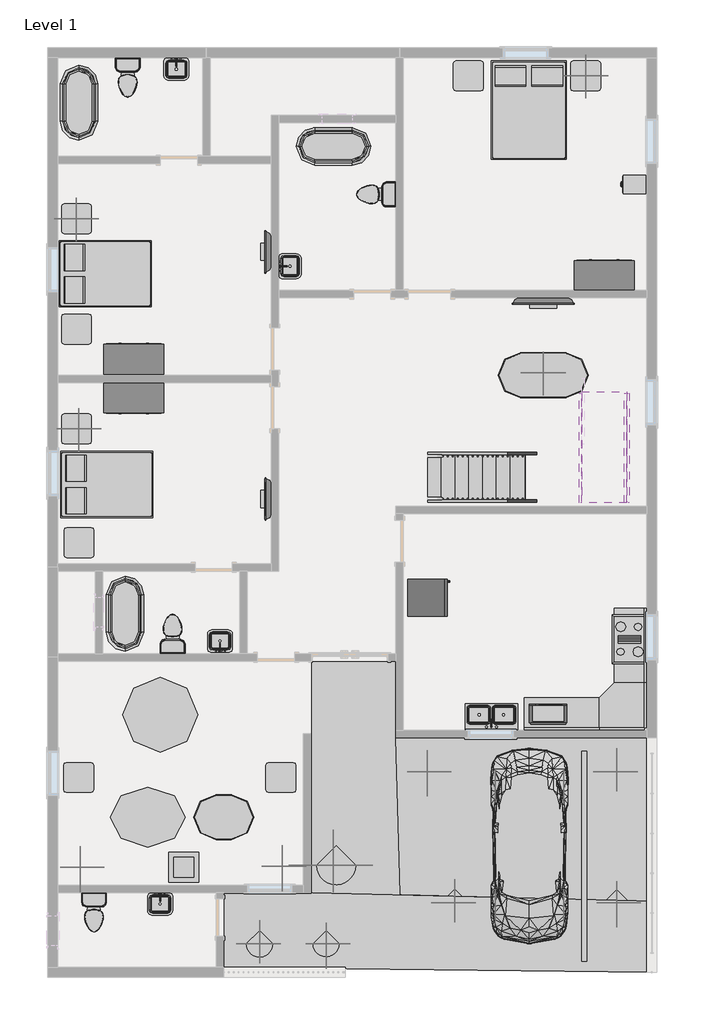
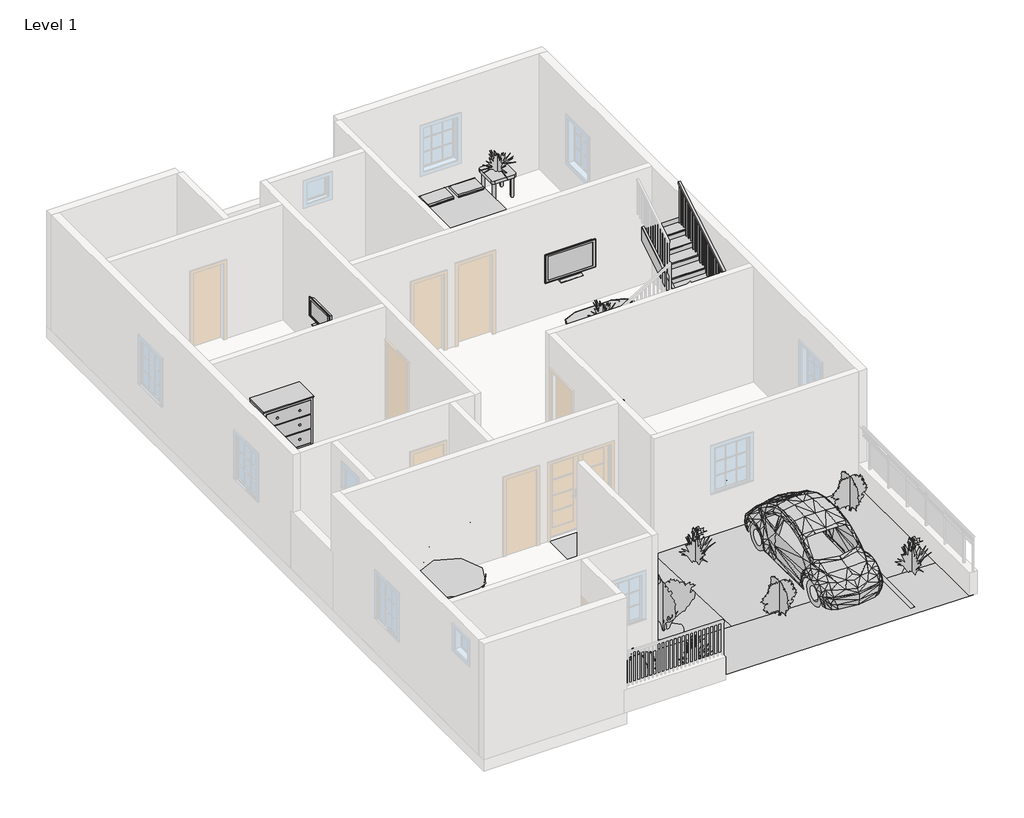
# One storey, part 3 of 3: 24 furniture elements, 16 flow terminals, 13 geographic elements, 8 proxies, 4 members, 2 stair flights, 1 railing.
"""IFC4 building model written with IfcOpenShell, lengths in millimetres."""

from ifc_helpers import new_model, si_unit, frame, origin, place, context, project, spatial, polyline, outline, extrude, triangles, transform, mapped, element, save
from components import proxy_bb1e6e30, proxy_8a8d5ab2, parking_space_9_x_18_90_deg_fdd9e8f5, rpc_beetle_rpc_beetle_3ce7ba48, proxy_a13a33b2, flow_terminal_accce45a, flow_terminal_a53be723, flow_terminal_62a433f7, toilet_domestic_3d_toilet_domestic_3d_f7549cf7, toilet_domestic_3d_toilet_domestic_3d_183bbd19, flow_terminal_b374fae2, furniture_c8abb964, furniture_1d2926bd, furniture_552c1472, furniture_9fa109b2, furniture_56245f3a, furniture_fdf74506, furniture_b5c51a22, furniture_be1c6672, furniture_2c34a4f9, furniture_bbcc68ce, furniture_743965d2, furniture_31d08a24, furniture_5c8231d0, rpc_plant_tropical_55f6ff97, rpc_plant_tropical_6475341c, rpc_plant_tropical_agave_1_5_93a2a214, rpc_plant_tropical_jungle_flame_3_9c4808c2, stair_flight_ef017676, stair_flight_8b003f58

model = new_model("IFC4")

# Units and contexts
model_context = context("Model", 3, world=origin())
ifc_project = project(units=[si_unit("LENGTHUNIT", "METRE", prefix="MILLI")], contexts=[model_context])

# Site, building, storey
site = spatial("IfcSite", under=ifc_project)
building = spatial("IfcBuilding", under=site)
storey = spatial("IfcBuildingStorey", under=building, Name="Level 1", Elevation=0.0)

# Proxies
placement = place(None, origin())
element("IfcBuildingElementProxy", 1, Name="Building Element Proxy", at=placement, inside=storey, context=model_context, shape_type="Tessellation", body=[
    triangles([(-8705.2791046, -6000.0233002, 0.0), (-8705.2791046, -7524.0233002, 0.0), (159.3210528, -7625.6229126, 0.0), (260.9210468, -6180.3093887, 0.0), (-6781.5930359, -6000.0233002, 0.0)], [[1, 2, 5], [5, 3, 4], [3, 5, 2]], closed=False),
])
element("IfcBuildingElementProxy", 2, Name="Building Element Proxy", at=placement, inside=storey, context=model_context, shape_type="Tessellation", body=[
    triangles([(-6774.8789108, -1287.4205452, 0.0), (-5200.0791046, -1287.4205452, 0.0), (-6781.5930359, -6000.0233002, 0.0), (-5203.2050766, -6030.7394485, 0.0), (-4939.7665054, -6039.441243, 0.0), (-4940.9478287, -6075.2140594, 0.0), (-5225.478717, -1169.9455936, 0.0), (-6736.7789108, -1204.8705694, 0.0), (-5047.6791046, -1287.4205452, 0.0), (-6784.7504013, -6048.9331055, 0.0)], [[10, 3, 1], [2, 1, 3], [8, 2, 7], [1, 2, 8], [3, 10, 4], [6, 5, 4], [4, 9, 2], [9, 4, 5], [2, 9, 7], [4, 2, 3], [6, 4, 10]], closed=False),
])
element("IfcBuildingElementProxy", 3, Name="Building Element Proxy", at=placement, inside=storey, context=model_context, shape_type="Tessellation", body=[
    triangles([(-5047.6791046, -2850.4231064, 0.0), (57.7210498, -2850.4231064, 0.0), (57.7210498, -6178.9426117, 0.0), (-4927.8021194, -6042.9741669, 0.0), (-4962.313385, -6033.9735535, 0.0)], [[1, 5, 4], [4, 3, 2], [4, 2, 1]], closed=False),
])
proxy_shape = proxy_bb1e6e30(model_context)
element("IfcBuildingElementProxy", 4, Name="Cook Top-4 Unit : 36\" x 20\"", ObjectType="Cook Top-4 Unit : 36\" x 20\"", at=placement, inside=storey, context=model_context, shape_type="MappedRepresentation", body=[
    mapped(proxy_shape, transform((-297.8789517, -843.8231522, 0.0), x_axis=(0.0, -1.0000000000000004, 0.0), y_axis=(1.0000000000000004, 0.0, 0.0), z_axis=(0.0, 0.0, 1.0))),
])
proxy_2_shape = proxy_8a8d5ab2(model_context)
element("IfcBuildingElementProxy", 5, Name="Microwave : 30\" x 16\" x 18\"", ObjectType="Microwave : 30\" x 16\" x 18\"", at=placement, inside=storey, context=model_context, shape_type="MappedRepresentation", body=[
    mapped(proxy_2_shape, transform((-1448.5860744, -2720.9036581, 0.0), x_axis=(-1.0000000000000004, 0.0, 0.0), y_axis=(0.0, -1.0000000000000004, 0.0), z_axis=(0.0, 0.0, 1.0))),
])
parking_space_9_x_18_90_deg_shape = parking_space_9_x_18_90_deg_fdd9e8f5(model_context)
element("IfcBuildingElementProxy", 6, Name="Parking Space : 9' x 18' - 90 deg", ObjectType="Parking Space : 9' x 18' - 90 deg", at=placement, inside=storey, context=model_context, shape_type="MappedRepresentation", body=[
    mapped(parking_space_9_x_18_90_deg_shape, transform((-1212.2789517, -7393.9424288, 0.0), x_axis=(-1.0000000000000004, 0.0, 0.0), y_axis=(0.0, -1.0000000000000004, 0.0), z_axis=(0.0, 0.0, 1.0))),
])
rpc_beetle_rpc_beetle_shape = rpc_beetle_rpc_beetle_3ce7ba48(model_context)
element("IfcBuildingElementProxy", 7, Name="RPC Beetle : RPC Beetle", ObjectType="RPC Beetle : RPC Beetle", at=placement, inside=storey, context=model_context, shape_type="MappedRepresentation", body=[
    mapped(rpc_beetle_rpc_beetle_shape, transform((-2329.8789517, -3815.6231522, 0.0), x_axis=(-1.0000000000000004, 0.0, 0.0), y_axis=(0.0, -1.0000000000000004, 0.0), z_axis=(0.0, 0.0, 1.0))),
])
proxy_3_shape = proxy_a13a33b2(model_context)
element("IfcBuildingElementProxy", 8, Name="Refrigerator : 30\" x 32\" RH", ObjectType="Refrigerator : 30\" x 32\" RH", at=placement, inside=storey, context=model_context, shape_type="MappedRepresentation", body=[
    mapped(proxy_3_shape, transform((-4420.6164517, 0.4304375, 0.0), x_axis=(0.0, 1.0000000000000002, 0.0), y_axis=(-1.0000000000000002, 0.0, 0.0), z_axis=(0.0, 0.0, 1.0))),
])

# Flow terminals
flow_terminal_shape = flow_terminal_accce45a(model_context)
element("IfcFlowTerminal", 9, ObjectType="Floor Drain - Round : 5\" Strainer - 2\" Drain", at=placement, inside=storey, context=model_context, shape_type="MappedRepresentation", body=[
    mapped(flow_terminal_shape, transform((-10889.6789517, 9290.7768478, 0.0), x_axis=(1.0, 0.0, 0.0), y_axis=(0.0, 1.0, 0.0), z_axis=(0.0, 0.0, 1.0))),
])
element("IfcFlowTerminal", 10, ObjectType="Floor Drain - Round : 5\" Strainer - 2\" Drain", at=placement, inside=storey, context=model_context, shape_type="MappedRepresentation", body=[
    mapped(flow_terminal_shape, transform((-7105.0789517, 8528.7768478, 0.0), x_axis=(1.0, 0.0, 0.0), y_axis=(0.0, 1.0, 0.0), z_axis=(0.0, 0.0, 1.0))),
])
element("IfcFlowTerminal", 11, ObjectType="Floor Drain - Round : 5\" Strainer - 2\" Drain", at=placement, inside=storey, context=model_context, shape_type="MappedRepresentation", body=[
    mapped(flow_terminal_shape, transform((-10051.4789517, 312.779409, 0.0), x_axis=(1.0, 0.0, 0.0), y_axis=(0.0, 1.0, 0.0), z_axis=(0.0, 0.0, 1.0))),
])
element("IfcFlowTerminal", 12, ObjectType="Floor Drain - Round : 5\" Strainer - 2\" Drain", at=placement, inside=storey, context=model_context, shape_type="MappedRepresentation", body=[
    mapped(flow_terminal_shape, transform((-11169.0789517, -7092.2231522, 0.0), x_axis=(1.0, 0.0, 0.0), y_axis=(0.0, 1.0, 0.0), z_axis=(0.0, 0.0, 1.0))),
])
flow_terminal_2_shape = flow_terminal_a53be723(model_context)
element("IfcFlowTerminal", 13, ObjectType="Sink Kitchen-Double : 42\" x 21\"", at=placement, inside=storey, context=model_context, shape_type="MappedRepresentation", body=[
    mapped(flow_terminal_2_shape, transform((-3088.8897111, -2416.2777511, 0.0), x_axis=(-1.0000000000000004, 0.0, 0.0), y_axis=(0.0, -1.0000000000000004, 0.0), z_axis=(0.0, 0.0, 1.0))),
])
flow_terminal_3_shape = flow_terminal_62a433f7(model_context)
element("IfcFlowTerminal", 14, ObjectType="Sink Vanity-Square : 20\" x 18\"", at=placement, inside=storey, context=model_context, shape_type="MappedRepresentation", body=[
    mapped(flow_terminal_3_shape, transform((-9533.7681923, 10812.4314467, 0.0), x_axis=(1.0, 0.0, 0.0), y_axis=(0.0, 1.0, 0.0), z_axis=(0.0, 0.0, 1.0))),
])
element("IfcFlowTerminal", 15, ObjectType="Sink Vanity-Square : 20\" x 18\"", at=placement, inside=storey, context=model_context, shape_type="MappedRepresentation", body=[
    mapped(flow_terminal_3_shape, transform((-7255.1335506, 6735.0876072, 0.0), x_axis=(0.0, 1.0000000000000002, 0.0), y_axis=(-1.0000000000000002, 0.0, 0.0), z_axis=(0.0, 0.0, 1.0))),
])
element("IfcFlowTerminal", 16, ObjectType="Sink Vanity-Square : 20\" x 18\"", at=placement, inside=storey, context=model_context, shape_type="MappedRepresentation", body=[
    mapped(flow_terminal_3_shape, transform((-8613.3897111, -929.4751899, 0.0), x_axis=(-1.0, 0.0, 0.0), y_axis=(0.0, -1.0, 0.0), z_axis=(0.0, 0.0, 1.0))),
])
element("IfcFlowTerminal", 17, ObjectType="Sink Vanity-Square : 20\" x 18\"", at=placement, inside=storey, context=model_context, shape_type="MappedRepresentation", body=[
    mapped(flow_terminal_3_shape, transform((-9863.9681923, -6180.1685533, 0.0), x_axis=(1.0, 0.0, 0.0), y_axis=(0.0, 1.0, 0.0), z_axis=(0.0, 0.0, 1.0))),
])
toilet_domestic_3d_toilet_domestic_3d_shape = toilet_domestic_3d_toilet_domestic_3d_f7549cf7(model_context)
toilet_domestic_3d_toilet_domestic_3d_2_shape = toilet_domestic_3d_toilet_domestic_3d_183bbd19(model_context)
element("IfcFlowTerminal", 18, ObjectType="Toilet-Domestic-3D : Toilet-Domestic-3D", at=placement, inside=storey, context=model_context, shape_type="MappedRepresentation", body=[
    mapped(toilet_domestic_3d_toilet_domestic_3d_shape, transform((-10508.6789517, 10497.8808204, 0.0), x_axis=(1.0, 0.0, 0.0), y_axis=(0.0, 1.0, 0.0), z_axis=(0.0, 0.0, 1.0))),
    mapped(toilet_domestic_3d_toilet_domestic_3d_2_shape, transform((-10508.6789517, 10497.8808204, 0.0), x_axis=(1.0, 0.0, 0.0), y_axis=(0.0, 1.0, 0.0), z_axis=(0.0, 0.0, 1.0))),
])
element("IfcFlowTerminal", 19, ObjectType="Toilet-Domestic-3D : Toilet-Domestic-3D", at=placement, inside=storey, context=model_context, shape_type="MappedRepresentation", body=[
    mapped(toilet_domestic_3d_toilet_domestic_3d_shape, transform((-5542.3749791, 8212.179409, 0.0), x_axis=(0.0, -1.0000000000000004, 0.0), y_axis=(1.0000000000000004, 0.0, 0.0), z_axis=(0.0, 0.0, 1.0))),
    mapped(toilet_domestic_3d_toilet_domestic_3d_2_shape, transform((-5542.3749791, 8212.179409, 0.0), x_axis=(0.0, -1.0000000000000004, 0.0), y_axis=(1.0000000000000004, 0.0, 0.0), z_axis=(0.0, 0.0, 1.0))),
])
element("IfcFlowTerminal", 20, ObjectType="Toilet-Domestic-3D : Toilet-Domestic-3D", at=placement, inside=storey, context=model_context, shape_type="MappedRepresentation", body=[
    mapped(toilet_domestic_3d_toilet_domestic_3d_shape, transform((-9594.2789517, -640.3245637, 0.0), x_axis=(-0.9999999999999999, 0.0, 0.0), y_axis=(0.0, -0.9999999999999999, 0.0), z_axis=(0.0, 0.0, 1.0))),
    mapped(toilet_domestic_3d_toilet_domestic_3d_2_shape, transform((-9594.2789517, -640.3245637, 0.0), x_axis=(-0.9999999999999999, 0.0, 0.0), y_axis=(0.0, -0.9999999999999999, 0.0), z_axis=(0.0, 0.0, 1.0))),
])
element("IfcFlowTerminal", 21, ObjectType="Toilet-Domestic-3D : Toilet-Domestic-3D", at=placement, inside=storey, context=model_context, shape_type="MappedRepresentation", body=[
    mapped(toilet_domestic_3d_toilet_domestic_3d_shape, transform((-11194.4789517, -6494.7191796, 0.0), x_axis=(1.0000000000000002, 0.0, 0.0), y_axis=(0.0, 1.0000000000000002, 0.0), z_axis=(0.0, 0.0, 1.0))),
    mapped(toilet_domestic_3d_toilet_domestic_3d_2_shape, transform((-11194.4789517, -6494.7191796, 0.0), x_axis=(1.0000000000000002, 0.0, 0.0), y_axis=(0.0, 1.0000000000000002, 0.0), z_axis=(0.0, 0.0, 1.0))),
])
flow_terminal_4_shape = flow_terminal_b374fae2(model_context)
element("IfcFlowTerminal", 22, ObjectType="Tub-Free Standing-3D : 30\" x 60\"", at=placement, inside=storey, context=model_context, shape_type="MappedRepresentation", body=[
    mapped(flow_terminal_4_shape, transform((-11499.2789517, 10078.1768478, 0.0), x_axis=(1.0, 0.0, 0.0), y_axis=(0.0, 1.0, 0.0), z_axis=(0.0, 0.0, 1.0))),
])
element("IfcFlowTerminal", 23, ObjectType="Tub-Free Standing-3D : 30\" x 60\"", at=placement, inside=storey, context=model_context, shape_type="MappedRepresentation", body=[
    mapped(flow_terminal_4_shape, transform((-6317.6789517, 9189.1768478, 0.0), x_axis=(0.0, 1.0000000000000002, 0.0), y_axis=(-1.0000000000000002, 0.0, 0.0), z_axis=(0.0, 0.0, 1.0))),
])
element("IfcFlowTerminal", 24, ObjectType="Tub-Free Standing-3D : 30\" x 60\"", at=placement, inside=storey, context=model_context, shape_type="MappedRepresentation", body=[
    mapped(flow_terminal_4_shape, transform((-10559.4789517, -322.220591, 0.0), x_axis=(1.0, 0.0, 0.0), y_axis=(0.0, 1.0, 0.0), z_axis=(0.0, 0.0, 1.0))),
])

# Furniture
furniture_shape = furniture_c8abb964(model_context)
element("IfcFurniture", 25, ObjectType="Bed-Box : Double 53\" x 74\"", at=placement, inside=storey, context=model_context, shape_type="MappedRepresentation", body=[
    mapped(furniture_shape, transform((-11200.3084599, 6256.379409, 0.0), x_axis=(0.0, 1.0, 0.0), y_axis=(-1.0, 0.0, 0.0), z_axis=(0.0, 0.0, 1.0))),
])
element("IfcFurniture", 26, ObjectType="Bed-Box : Double 53\" x 74\"", at=placement, inside=storey, context=model_context, shape_type="MappedRepresentation", body=[
    mapped(furniture_shape, transform((-11169.0789517, 1967.52695, 0.0), x_axis=(0.0, 1.0, 0.0), y_axis=(-1.0, 0.0, 0.0), z_axis=(0.0, 0.0, 1.0))),
])
furniture_2_shape = furniture_1d2926bd(model_context)
element("IfcFurniture", 27, ObjectType="Bed-Box : Queen 60\" x 79\"", at=placement, inside=storey, context=model_context, shape_type="MappedRepresentation", body=[
    mapped(furniture_2_shape, transform((-2681.7314107, 10160.206356, 0.0), x_axis=(1.0, 0.0, 0.0), y_axis=(0.0, 1.0, 0.0), z_axis=(0.0, 0.0, 1.0))),
])
furniture_3_shape = furniture_552c1472(model_context)
element("IfcFurniture", 28, ObjectType="Cabinet-File 3 Drawer : 15\" x 18\"", at=placement, inside=storey, context=model_context, shape_type="MappedRepresentation", body=[
    mapped(furniture_3_shape, transform((-54.1446516, 8286.5804007, 0.0), x_axis=(0.0, -1.0, 0.0), y_axis=(1.0, 0.0, 0.0), z_axis=(0.0, 0.0, 1.0))),
])
furniture_4_shape = furniture_9fa109b2(model_context)
element("IfcFurniture", 29, ObjectType="Dresser : 48\" x 72\" x 24\"", at=placement, inside=storey, context=model_context, shape_type="MappedRepresentation", body=[
    mapped(furniture_4_shape, transform((-10112.4856919, 4435.1423631, 0.0), x_axis=(1.0, 0.0, 0.0), y_axis=(0.0, 1.0, 0.0), z_axis=(0.0, 0.0, 1.0))),
])
element("IfcFurniture", 30, ObjectType="Dresser : 48\" x 72\" x 24\"", at=placement, inside=storey, context=model_context, shape_type="MappedRepresentation", body=[
    mapped(furniture_4_shape, transform((-10650.8722115, 4496.2164549, 0.0), x_axis=(-1.0000000000000002, 0.0, 0.0), y_axis=(0.0, -1.0000000000000002, 0.0), z_axis=(0.0, 0.0, 1.0))),
])
element("IfcFurniture", 31, ObjectType="Dresser : 48\" x 72\" x 24\"", at=placement, inside=storey, context=model_context, shape_type="MappedRepresentation", body=[
    mapped(furniture_4_shape, transform((-1075.0722115, 6198.0164549, 0.0), x_axis=(-1.0000000000000004, 0.0, 0.0), y_axis=(0.0, -1.0000000000000004, 0.0), z_axis=(0.0, 0.0, 1.0))),
])
furniture_5_shape = furniture_56245f3a(model_context)
element("IfcFurniture", 32, ObjectType="TV - Flat Screen : 32\"", at=placement, inside=storey, context=model_context, shape_type="MappedRepresentation", body=[
    mapped(furniture_5_shape, transform((-7648.2698861, 7039.8348948, 914.4), x_axis=(0.0, -1.0000000000000004, 0.0), y_axis=(1.0000000000000004, 0.0, 0.0), z_axis=(0.0, 0.0, 1.0))),
])
element("IfcFurniture", 33, ObjectType="TV - Flat Screen : 32\"", at=placement, inside=storey, context=model_context, shape_type="MappedRepresentation", body=[
    mapped(furniture_5_shape, transform((-7646.2175754, 2010.6348948, 914.4), x_axis=(0.0, -1.0000000000000004, 0.0), y_axis=(1.0000000000000004, 0.0, 0.0), z_axis=(0.0, 0.0, 1.0))),
])
furniture_6_shape = furniture_fdf74506(model_context)
element("IfcFurniture", 34, ObjectType="TV - Flat Screen : 50\"", at=placement, inside=storey, context=model_context, shape_type="MappedRepresentation", body=[
    mapped(furniture_6_shape, transform((-2046.5344376, 6045.4407853, 914.4), x_axis=(1.0, 0.0, 0.0), y_axis=(0.0, 1.0, 0.0), z_axis=(0.0, 0.0, 1.0))),
])
furniture_7_shape = furniture_b5c51a22(model_context)
element("IfcFurniture", 35, ObjectType="Table-Coffee : 24\" x 24\" x 24\"", at=placement, inside=storey, context=model_context, shape_type="MappedRepresentation", body=[
    mapped(furniture_7_shape, transform((-9383.9447184, -5580.88423, 0.0), x_axis=(1.0, 0.0, 0.0), y_axis=(0.0, 1.0, 0.0), z_axis=(0.0, 0.0, 1.0))),
])
furniture_8_shape = furniture_be1c6672(model_context)
element("IfcFurniture", 36, ObjectType="Table-Dining Oval : 36\" x 48\"", at=placement, inside=storey, context=model_context, shape_type="MappedRepresentation", body=[
    mapped(furniture_8_shape, transform((-8151.0592796, -4104.3222304, 0.0), x_axis=(1.0, 0.0, 0.0), y_axis=(0.0, 1.0, 0.0), z_axis=(0.0, 0.0, 1.0))),
])
furniture_9_shape = furniture_2c34a4f9(model_context)
element("IfcFurniture", 37, ObjectType="Table-Dining Oval : 36\" x 72\"", at=placement, inside=storey, context=model_context, shape_type="MappedRepresentation", body=[
    mapped(furniture_9_shape, transform((-1648.6592796, 4887.2777696, 0.0), x_axis=(1.0, 0.0, 0.0), y_axis=(0.0, 1.0, 0.0), z_axis=(0.0, 0.0, 1.0))),
])
furniture_10_shape = furniture_bbcc68ce(model_context)
element("IfcFurniture", 38, ObjectType="Table-Dining Round w Chairs : 60\" Diameter", at=placement, inside=storey, context=model_context, shape_type="MappedRepresentation", body=[
    mapped(furniture_10_shape, transform((-9951.9609189, -2194.7419025, 0.0), x_axis=(1.0, 0.0, 0.0), y_axis=(0.0, 1.0, 0.0), z_axis=(0.0, 0.0, 1.0))),
])
furniture_11_shape = furniture_743965d2(model_context)
element("IfcFurniture", 39, ObjectType="Table-Ellipse : 60\" x 48\"", at=placement, inside=storey, context=model_context, shape_type="MappedRepresentation", body=[
    mapped(furniture_11_shape, transform((-10102.2789517, -4462.420591, 0.0), x_axis=(1.0, 0.0, 0.0), y_axis=(0.0, 1.0, 0.0), z_axis=(0.0, 0.0, 1.0))),
])
furniture_12_shape = furniture_31d08a24(model_context)
element("IfcFurniture", 40, ObjectType="Table-End : 24\" x 24\"", at=placement, inside=storey, context=model_context, shape_type="MappedRepresentation", body=[
    mapped(furniture_12_shape, transform((-11858.612582, 7563.5768478, 0.0), x_axis=(1.0, 0.0, 0.0), y_axis=(0.0, 1.0, 0.0), z_axis=(0.0, 0.0, 1.0))),
])
element("IfcFurniture", 41, ObjectType="Table-End : 24\" x 24\"", at=placement, inside=storey, context=model_context, shape_type="MappedRepresentation", body=[
    mapped(furniture_12_shape, transform((-11858.612582, 5316.579409, 0.0), x_axis=(1.0, 0.0, 0.0), y_axis=(0.0, 1.0, 0.0), z_axis=(0.0, 0.0, 1.0))),
])
element("IfcFurniture", 42, ObjectType="Table-End : 24\" x 24\"", at=placement, inside=storey, context=model_context, shape_type="MappedRepresentation", body=[
    mapped(furniture_12_shape, transform((-11807.812582, 973.179409, 0.0), x_axis=(1.0, 0.0, 0.0), y_axis=(0.0, 1.0, 0.0), z_axis=(0.0, 0.0, 1.0))),
])
element("IfcFurniture", 43, ObjectType="Table-End : 24\" x 24\"", at=placement, inside=storey, context=model_context, shape_type="MappedRepresentation", body=[
    mapped(furniture_12_shape, transform((-11858.612582, 3284.579409, 0.0), x_axis=(1.0, 0.0, 0.0), y_axis=(0.0, 1.0, 0.0), z_axis=(0.0, 0.0, 1.0))),
])
element("IfcFurniture", 44, ObjectType="Table-End : 24\" x 24\"", at=placement, inside=storey, context=model_context, shape_type="MappedRepresentation", body=[
    mapped(furniture_12_shape, transform((-11814.5264088, -3809.2731522, 0.0), x_axis=(1.0, 0.0, 0.0), y_axis=(0.0, 1.0, 0.0), z_axis=(0.0, 0.0, 1.0))),
])
element("IfcFurniture", 45, ObjectType="Table-End : 24\" x 24\"", at=placement, inside=storey, context=model_context, shape_type="MappedRepresentation", body=[
    mapped(furniture_12_shape, transform((-7699.7264088, -3809.2731522, 0.0), x_axis=(1.0, 0.0, 0.0), y_axis=(0.0, 1.0, 0.0), z_axis=(0.0, 0.0, 1.0))),
])
element("IfcFurniture", 46, ObjectType="Table-End : 24\" x 24\"", at=placement, inside=storey, context=model_context, shape_type="MappedRepresentation", body=[
    mapped(furniture_12_shape, transform((-1495.412582, 10471.8768478, 0.0), x_axis=(1.0, 0.0, 0.0), y_axis=(0.0, 1.0, 0.0), z_axis=(0.0, 0.0, 1.0))),
])
element("IfcFurniture", 47, ObjectType="Table-End : 24\" x 24\"", at=placement, inside=storey, context=model_context, shape_type="MappedRepresentation", body=[
    mapped(furniture_12_shape, transform((-3883.012582, 10471.8768478, 0.0), x_axis=(1.0, 0.0, 0.0), y_axis=(0.0, 1.0, 0.0), z_axis=(0.0, 0.0, 1.0))),
])
furniture_13_shape = furniture_5c8231d0(model_context)
element("IfcFurniture", 48, ObjectType="Work Station Cubicle : 96\" x 96\"", at=placement, inside=storey, context=model_context, shape_type="MappedRepresentation", body=[
    mapped(furniture_13_shape, transform((-74.0107039, -3193.0461599, 0.0), x_axis=(-1.0000000000000004, 0.0, 0.0), y_axis=(0.0, -1.0000000000000004, 0.0), z_axis=(0.0, 0.0, 1.0))),
])

# Geographic elements
rpc_plant_tropical_shape = rpc_plant_tropical_55f6ff97(model_context)
element("IfcGeographicElement", 49, ObjectType="RPC Plant - Tropical", at=placement, inside=storey, context=model_context, shape_type="MappedRepresentation", body=[
    mapped(rpc_plant_tropical_shape, transform((-11473.8789517, -5485.6731522, 0.0), x_axis=(1.0, 0.0, 0.0), y_axis=(0.0, 1.0, 0.0), z_axis=(0.0, 0.0, 1.0))),
])
element("IfcGeographicElement", 50, ObjectType="RPC Plant - Tropical", at=placement, inside=storey, context=model_context, shape_type="MappedRepresentation", body=[
    mapped(rpc_plant_tropical_shape, transform((-7365.7927785, -5463.5424288, 0.0), x_axis=(1.0, 0.0, 0.0), y_axis=(0.0, 1.0, 0.0), z_axis=(0.0, 0.0, 1.0))),
])
element("IfcGeographicElement", 51, ObjectType="RPC Plant - Tropical", at=placement, inside=storey, context=model_context, shape_type="MappedRepresentation", body=[
    mapped(rpc_plant_tropical_shape, transform((-4412.6789517, -3536.2231522, 0.0), x_axis=(1.0, 0.0, 0.0), y_axis=(0.0, 1.0, 0.0), z_axis=(0.0, 0.0, 1.0))),
])
element("IfcGeographicElement", 52, ObjectType="RPC Plant - Tropical", at=placement, inside=storey, context=model_context, shape_type="MappedRepresentation", body=[
    mapped(rpc_plant_tropical_shape, transform((-551.8789517, -6203.2231522, 0.0), x_axis=(1.0, 0.0, 0.0), y_axis=(0.0, 1.0, 0.0), z_axis=(0.0, 0.0, 1.0))),
])
element("IfcGeographicElement", 53, ObjectType="RPC Plant - Tropical", at=placement, inside=storey, context=model_context, shape_type="MappedRepresentation", body=[
    mapped(rpc_plant_tropical_shape, transform((-6470.0789517, -7041.4231522, 0.0), x_axis=(1.0, 0.0, 0.0), y_axis=(0.0, 1.0, 0.0), z_axis=(0.0, 0.0, 1.0))),
])
rpc_plant_tropical_2_shape = rpc_plant_tropical_6475341c(model_context)
element("IfcGeographicElement", 54, ObjectType="RPC Plant - Tropical", at=placement, inside=storey, context=model_context, shape_type="MappedRepresentation", body=[
    mapped(rpc_plant_tropical_2_shape, transform((-6266.8789517, -5441.2231522, 0.0), x_axis=(1.0, 0.0, 0.0), y_axis=(0.0, 1.0, 0.0), z_axis=(0.0, 0.0, 1.0))),
])
rpc_plant_tropical_agave_1_5_shape = rpc_plant_tropical_agave_1_5_93a2a214(model_context)
element("IfcGeographicElement", 55, ObjectType="RPC Plant - Tropical : Agave - 1.5'", at=placement, inside=storey, context=model_context, shape_type="MappedRepresentation", body=[
    mapped(rpc_plant_tropical_agave_1_5_shape, transform((-11550.0789517, 7715.9768478, 609.6), x_axis=(1.0, 0.0, 0.0), y_axis=(0.0, 1.0, 0.0), z_axis=(0.0, 0.0, 1.0))),
])
element("IfcGeographicElement", 56, ObjectType="RPC Plant - Tropical : Agave - 1.5'", at=placement, inside=storey, context=model_context, shape_type="MappedRepresentation", body=[
    mapped(rpc_plant_tropical_agave_1_5_shape, transform((-11499.2789517, 3436.979409, 609.6), x_axis=(1.0, 0.0, 0.0), y_axis=(0.0, 1.0, 0.0), z_axis=(0.0, 0.0, 1.0))),
])
element("IfcGeographicElement", 57, ObjectType="RPC Plant - Tropical : Agave - 1.5'", at=placement, inside=storey, context=model_context, shape_type="MappedRepresentation", body=[
    mapped(rpc_plant_tropical_agave_1_5_shape, transform((-2050.4789517, 4579.979409, 609.6), x_axis=(1.0, 0.0, 0.0), y_axis=(0.0, 1.0, 0.0), z_axis=(0.0, 0.0, 1.0))),
])
element("IfcGeographicElement", 58, ObjectType="RPC Plant - Tropical : Agave - 1.5'", at=placement, inside=storey, context=model_context, shape_type="MappedRepresentation", body=[
    mapped(rpc_plant_tropical_agave_1_5_shape, transform((-1186.8789517, 10624.2768478, 609.6), x_axis=(1.0, 0.0, 0.0), y_axis=(0.0, 1.0, 0.0), z_axis=(0.0, 0.0, 1.0))),
])
rpc_plant_tropical_jungle_flame_3_shape = rpc_plant_tropical_jungle_flame_3_9c4808c2(model_context)
element("IfcGeographicElement", 59, ObjectType="RPC Plant - Tropical : Jungle Flame - 3'", at=placement, inside=storey, context=model_context, shape_type="MappedRepresentation", body=[
    mapped(rpc_plant_tropical_jungle_flame_3_shape, transform((-7822.9927785, -7041.4231522, 0.0), x_axis=(1.0, 0.0, 0.0), y_axis=(0.0, 1.0, 0.0), z_axis=(0.0, 0.0, 1.0))),
])
element("IfcGeographicElement", 60, ObjectType="RPC Plant - Tropical : Jungle Flame - 3'", at=placement, inside=storey, context=model_context, shape_type="MappedRepresentation", body=[
    mapped(rpc_plant_tropical_jungle_flame_3_shape, transform((-3853.8789517, -6203.2231522, 0.0), x_axis=(1.0, 0.0, 0.0), y_axis=(0.0, 1.0, 0.0), z_axis=(0.0, 0.0, 1.0))),
])
element("IfcGeographicElement", 61, ObjectType="RPC Plant - Tropical : Jungle Flame - 3'", at=placement, inside=storey, context=model_context, shape_type="MappedRepresentation", body=[
    mapped(rpc_plant_tropical_jungle_flame_3_shape, transform((-551.8789517, -3536.2231522, 0.0), x_axis=(1.0, 0.0, 0.0), y_axis=(0.0, 1.0, 0.0), z_axis=(0.0, 0.0, 1.0))),
])

# Members
element("IfcMember", 62, ObjectType="Stringer - 2\" Width", at=placement, inside=storey, context=model_context, shape_type="SweptSolid", body=[
    extrude(outline(polyline([(212.114512, -4400.7663486), (0.0, -4400.7663486), (0.0, -4162.6808368), (1718.3724171, -1327.3663486), (2074.7811786, -1327.3663486), (212.114512, -4400.7663486)])), frame((0.0, 2907.7117215, 0.0), z_axis=(0.0, 1.0, 0.0), x_axis=(0.0, 0.0, 1.0)), (0.0, 0.0, 1.0), 50.8),
])
element("IfcMember", 63, ObjectType="Stringer - 2\" Width", at=placement, inside=storey, context=model_context, shape_type="SweptSolid", body=[
    extrude(outline(polyline([(212.114512, -4400.7663486), (0.0, -4400.7663486), (0.0, -4162.6808368), (1718.3724171, -1327.3663486), (2074.7811786, -1327.3663486), (212.114512, -4400.7663486)])), frame((0.0, 1942.5117215, 0.0), z_axis=(0.0, 1.0, 0.0), x_axis=(0.0, 0.0, 1.0)), (0.0, 0.0, 1.0), 50.8),
])
element("IfcMember", 64, ObjectType="Stringer - 2\" Width", at=placement, inside=storey, context=model_context, shape_type="SweptSolid", body=[
    extrude(outline(polyline([(1930.818583, 1379.7057504), (1930.818583, 1736.114512), (4166.018583, 3090.7811786), (4166.018583, 2734.3724171), (1930.818583, 1379.7057504)])), frame((-1313.8789517, 0.0, 0.0), z_axis=(1.0, 0.0, 0.0), x_axis=(0.0, 1.0, 0.0)), (0.0, 0.0, 1.0), 50.8),
])
element("IfcMember", 65, ObjectType="Stringer - 2\" Width", at=placement, inside=storey, context=model_context, shape_type="SweptSolid", body=[
    extrude(outline(polyline([(1930.818583, 1379.7057504), (1930.818583, 1736.114512), (4166.018583, 3090.7811786), (4166.018583, 2734.3724171), (1930.818583, 1379.7057504)])), frame((-348.6789517, 0.0, 0.0), z_axis=(1.0, 0.0, 0.0), x_axis=(0.0, 1.0, 0.0)), (0.0, 0.0, 1.0), 50.8),
])

# Railing
element("IfcRailing", 66, ObjectType="Handrail - Rectangular", at=placement, inside=storey, context=model_context, shape_type="SweptSolid", body=[
    extrude(outline(polyline([(1930.818583, 2548.3318731), (1930.818583, 2607.7333333), (4166.018583, 3962.4), (4166.018583, 3902.9985397), (1930.818583, 2548.3318731)])), frame((-399.4789517, 0.0, 0.0), z_axis=(1.0, 0.0, 0.0), x_axis=(0.0, 1.0, 0.0)), (0.0, 0.0, 1.0), 50.8),
    extrude(outline(polyline([(2041.943583, 2615.6803579), (2041.943583, 1693.3333333), (2022.893583, 1693.3333333), (2022.893583, 2604.1349034), (2041.943583, 2615.6803579)])), frame((-383.6039517, 0.0, 0.0), z_axis=(1.0, 0.0, 0.0), x_axis=(0.0, 1.0, 0.0)), (0.0, 0.0, 1.0), 19.05),
    extrude(outline(polyline([(2143.543583, 2677.2561155), (2143.543583, 1693.3333333), (2124.493583, 1693.3333333), (2124.493583, 2665.710661), (2143.543583, 2677.2561155)])), frame((-383.6039517, 0.0, 0.0), z_axis=(1.0, 0.0, 0.0), x_axis=(0.0, 1.0, 0.0)), (0.0, 0.0, 1.0), 19.05),
    extrude(outline(polyline([(2245.143583, 2738.8318731), (2245.143583, 1862.6666667), (2226.093583, 1862.6666667), (2226.093583, 2727.2864185), (2245.143583, 2738.8318731)])), frame((-383.6039517, 0.0, 0.0), z_axis=(1.0, 0.0, 0.0), x_axis=(0.0, 1.0, 0.0)), (0.0, 0.0, 1.0), 19.05),
    extrude(outline(polyline([(2346.743583, 2800.4076307), (2346.743583, 1862.6666667), (2327.693583, 1862.6666667), (2327.693583, 2788.8621761), (2346.743583, 2800.4076307)])), frame((-383.6039517, 0.0, 0.0), z_axis=(1.0, 0.0, 0.0), x_axis=(0.0, 1.0, 0.0)), (0.0, 0.0, 1.0), 19.05),
    extrude(outline(polyline([(2448.343583, 2861.9833882), (2448.343583, 1862.6666667), (2429.293583, 1862.6666667), (2429.293583, 2850.4379337), (2448.343583, 2861.9833882)])), frame((-383.6039517, 0.0, 0.0), z_axis=(1.0, 0.0, 0.0), x_axis=(0.0, 1.0, 0.0)), (0.0, 0.0, 1.0), 19.05),
    extrude(outline(polyline([(2549.943583, 2923.5591458), (2549.943583, 2032.0), (2530.893583, 2032.0), (2530.893583, 2912.0136913), (2549.943583, 2923.5591458)])), frame((-383.6039517, 0.0, 0.0), z_axis=(1.0, 0.0, 0.0), x_axis=(0.0, 1.0, 0.0)), (0.0, 0.0, 1.0), 19.05),
    extrude(outline(polyline([(2651.543583, 2985.1349034), (2651.543583, 2032.0), (2632.493583, 2032.0), (2632.493583, 2973.5894488), (2651.543583, 2985.1349034)])), frame((-383.6039517, 0.0, 0.0), z_axis=(1.0, 0.0, 0.0), x_axis=(0.0, 1.0, 0.0)), (0.0, 0.0, 1.0), 19.05),
    extrude(outline(polyline([(2753.143583, 3046.710661), (2753.143583, 2032.0), (2734.093583, 2032.0), (2734.093583, 3035.1652064), (2753.143583, 3046.710661)])), frame((-383.6039517, 0.0, 0.0), z_axis=(1.0, 0.0, 0.0), x_axis=(0.0, 1.0, 0.0)), (0.0, 0.0, 1.0), 19.05),
    extrude(outline(polyline([(2854.743583, 3108.2864185), (2854.743583, 2201.3333333), (2835.693583, 2201.3333333), (2835.693583, 3096.740964), (2854.743583, 3108.2864185)])), frame((-383.6039517, 0.0, 0.0), z_axis=(1.0, 0.0, 0.0), x_axis=(0.0, 1.0, 0.0)), (0.0, 0.0, 1.0), 19.05),
    extrude(outline(polyline([(2956.343583, 3169.8621761), (2956.343583, 2201.3333333), (2937.293583, 2201.3333333), (2937.293583, 3158.3167216), (2956.343583, 3169.8621761)])), frame((-383.6039517, 0.0, 0.0), z_axis=(1.0, 0.0, 0.0), x_axis=(0.0, 1.0, 0.0)), (0.0, 0.0, 1.0), 19.05),
    extrude(outline(polyline([(3057.943583, 3231.4379337), (3057.943583, 2370.6666667), (3038.893583, 2370.6666667), (3038.893583, 3219.8924791), (3057.943583, 3231.4379337)])), frame((-383.6039517, 0.0, 0.0), z_axis=(1.0, 0.0, 0.0), x_axis=(0.0, 1.0, 0.0)), (0.0, 0.0, 1.0), 19.05),
    extrude(outline(polyline([(3159.543583, 3293.0136913), (3159.543583, 2370.6666667), (3140.493583, 2370.6666667), (3140.493583, 3281.4682367), (3159.543583, 3293.0136913)])), frame((-383.6039517, 0.0, 0.0), z_axis=(1.0, 0.0, 0.0), x_axis=(0.0, 1.0, 0.0)), (0.0, 0.0, 1.0), 19.05),
    extrude(outline(polyline([(3261.143583, 3354.5894488), (3261.143583, 2370.6666667), (3242.093583, 2370.6666667), (3242.093583, 3343.0439943), (3261.143583, 3354.5894488)])), frame((-383.6039517, 0.0, 0.0), z_axis=(1.0, 0.0, 0.0), x_axis=(0.0, 1.0, 0.0)), (0.0, 0.0, 1.0), 19.05),
    extrude(outline(polyline([(3362.743583, 3416.1652064), (3362.743583, 2540.0), (3343.693583, 2540.0), (3343.693583, 3404.6197519), (3362.743583, 3416.1652064)])), frame((-383.6039517, 0.0, 0.0), z_axis=(1.0, 0.0, 0.0), x_axis=(0.0, 1.0, 0.0)), (0.0, 0.0, 1.0), 19.05),
    extrude(outline(polyline([(3464.343583, 3477.740964), (3464.343583, 2540.0), (3445.293583, 2540.0), (3445.293583, 3466.1955094), (3464.343583, 3477.740964)])), frame((-383.6039517, 0.0, 0.0), z_axis=(1.0, 0.0, 0.0), x_axis=(0.0, 1.0, 0.0)), (0.0, 0.0, 1.0), 19.05),
    extrude(outline(polyline([(3565.943583, 3539.3167216), (3565.943583, 2540.0), (3546.893583, 2540.0), (3546.893583, 3527.771267), (3565.943583, 3539.3167216)])), frame((-383.6039517, 0.0, 0.0), z_axis=(1.0, 0.0, 0.0), x_axis=(0.0, 1.0, 0.0)), (0.0, 0.0, 1.0), 19.05),
    extrude(outline(polyline([(3667.543583, 3600.8924791), (3667.543583, 2709.3333333), (3648.493583, 2709.3333333), (3648.493583, 3589.3470246), (3667.543583, 3600.8924791)])), frame((-383.6039517, 0.0, 0.0), z_axis=(1.0, 0.0, 0.0), x_axis=(0.0, 1.0, 0.0)), (0.0, 0.0, 1.0), 19.05),
    extrude(outline(polyline([(3769.143583, 3662.4682367), (3769.143583, 2709.3333333), (3750.093583, 2709.3333333), (3750.093583, 3650.9227822), (3769.143583, 3662.4682367)])), frame((-383.6039517, 0.0, 0.0), z_axis=(1.0, 0.0, 0.0), x_axis=(0.0, 1.0, 0.0)), (0.0, 0.0, 1.0), 19.05),
    extrude(outline(polyline([(3870.743583, 3724.0439943), (3870.743583, 2709.3333333), (3851.693583, 2709.3333333), (3851.693583, 3712.4985397), (3870.743583, 3724.0439943)])), frame((-383.6039517, 0.0, 0.0), z_axis=(1.0, 0.0, 0.0), x_axis=(0.0, 1.0, 0.0)), (0.0, 0.0, 1.0), 19.05),
    extrude(outline(polyline([(3972.343583, 3785.6197519), (3972.343583, 2878.6666667), (3953.293583, 2878.6666667), (3953.293583, 3774.0742973), (3972.343583, 3785.6197519)])), frame((-383.6039517, 0.0, 0.0), z_axis=(1.0, 0.0, 0.0), x_axis=(0.0, 1.0, 0.0)), (0.0, 0.0, 1.0), 19.05),
    extrude(outline(polyline([(4073.943583, 3847.1955094), (4073.943583, 2878.6666667), (4054.893583, 2878.6666667), (4054.893583, 3835.6500549), (4073.943583, 3847.1955094)])), frame((-383.6039517, 0.0, 0.0), z_axis=(1.0, 0.0, 0.0), x_axis=(0.0, 1.0, 0.0)), (0.0, 0.0, 1.0), 19.05),
    extrude(outline(polyline([(1949.868583, 2559.8773276), (1949.868583, 1693.3333333), (1930.818583, 1693.3333333), (1930.818583, 2548.3318731), (1949.868583, 2559.8773276)])), frame((-383.6039517, 0.0, 0.0), z_axis=(1.0, 0.0, 0.0), x_axis=(0.0, 1.0, 0.0)), (0.0, 0.0, 1.0), 19.05),
    extrude(outline(polyline([(4166.018583, 3902.9985397), (4166.018583, 2878.6666667), (4146.968583, 2878.6666667), (4146.968583, 3891.4530852), (4166.018583, 3902.9985397)])), frame((-383.6039517, 0.0, 0.0), z_axis=(1.0, 0.0, 0.0), x_axis=(0.0, 1.0, 0.0)), (0.0, 0.0, 1.0), 19.05),
])

# Stair flights
stair_flight_shape = stair_flight_ef017676(model_context)
element("IfcStairFlight", 67, ObjectType="2\" Tread 1\" Nosing 1/4\" Riser", at=placement, inside=storey, context=model_context, shape_type="MappedRepresentation", body=[
    mapped(stair_flight_shape, transform((0.0, 0.0, 0.0), x_axis=(1.0, 0.0, 0.0), y_axis=(0.0, 1.0, 0.0), z_axis=(0.0, 0.0, 1.0))),
])
stair_flight_2_shape = stair_flight_8b003f58(model_context)
element("IfcStairFlight", 68, ObjectType="2\" Tread 1\" Nosing 1/4\" Riser", at=placement, inside=storey, context=model_context, shape_type="MappedRepresentation", body=[
    mapped(stair_flight_2_shape, transform((0.0, 0.0, 0.0), x_axis=(1.0, 0.0, 0.0), y_axis=(0.0, 1.0, 0.0), z_axis=(0.0, 0.0, 1.0))),
])

save(model, "model.ifc")

# Revit data of these elements
# Type "Cook Top-4 Unit : 36\" x 20\""
#   Assembly Code = "E1090400"
#   Depth = 2' - 0"
#   Width = 3' - 0"
#   Burner Material = Steel, Chrome Plated
#   Cooktop Material = Steel, Polished
#   Default Elevation = 0
# Type "Microwave : 30\" x 16\" x 18\""
#   Assembly Code = "E1090400"
#   Depth = 1' - 4"
#   Height = 1' - 6"
#   Width = 2' - 6"
#   Microwave Material = Laminate, Ivory, Matte
#   Default Elevation = 0
# Type "Parking Space : 9' x 18' - 90 deg"
#   Angle = 90.00°
#   Parking Length = 18' - 0"
#   Parking Width = 9' - 0"
#   pl = 14' - 0"
#   pw = 7' - 0"
# Type "RPC Beetle : RPC Beetle"
#   built-in parameter 1005195 = "RPC-16-0U6E-L4EG-ENH1-J3KF-SVEL-0TX4-C0"
#   Height = 0
# Type "Refrigerator : 30\" x 32\" RH"
#   Label = "REF."
#   Assembly Code = "E1090400"
#   Depth = 2' - 7 3/4"
#   Handle = 2' - 3"
#   Height = 5' - 10"
#   Rear Clearance = 0' - 2"
#   Top Door Height = 1' - 8"
#   Width = 2' - 5 3/8"
#   Material = Steel, Paint Finish, Ivory, Glossy
#   Default Elevation = 0
# Type "Floor Drain - Round : 5\" Strainer - 2\" Drain"
#   WFU = 2
#   Strainer Height = 0' - 3 1/4"
#   Strainer Radius = 0' - 2 1/2"
#   Strainer Diameter = 0' - 5"
#   Radius 6 = 0' - 0 5/8"
#   Radius 5 = 0' - 1 1/4"
#   Radius 4 = 0' - 1 7/8"
#   Radius 2 = 0' - 3.04167"
#   Radius 1 = 0' - 2.02083"
#   Radius 3 = 0' - 2 1/32"
#   Pipe Radius = 1"
#   Pipe Diameter = 2"
#   Height 2 = 0' - 0.725"
#   Height 1 = 0' - 1 13/16"
#   Body Radius = 0' - 4 1/16"
#   Body Height = 0' - 3 5/8"
#   Body Diameter = 0' - 8 1/8"
#   Drain Material = none
#   HWFU = 0
#   Default Elevation = 0
#   CWFU = 0
# Type "Sink Kitchen-Double : 42\" x 21\""
#   Assembly Code = "D2010410"
#   Counter Height = 3' - 0"
#   Depth = 1' - 9"
#   Width = 3' - 6"
#   Faucet Material = Steel, Polished
#   Sink Material = Steel, Polished
#   Default Elevation = 0
# Type "Sink Vanity-Square : 20\" x 18\""
#   Assembly Code = "D2010400"
#   Counter Height = 2' - 7"
#   Depth = 1' - 6"
#   Width = 1' - 8"
#   Basin Material = Porcelain, Linen
#   Faucet Material = Steel, Polished
#   Default Elevation = 0
# Type "Toilet-Domestic-3D : Toilet-Domestic-3D"
#   Assembly Code = "D2010110"
#   Toilet - Bowl/Basin Material = Porcelain, Linen
#   Toilet - Seat Material = Laminate, Linen, Matte
#   Default Elevation = 0
# Type "Tub-Free Standing-3D : 30\" x 60\""
#   Assembly Code = "D2010110"
#   Height = 1' - 6"
#   Length = 5' - 0"
#   Width = 2' - 6"
#   Tub Material = Porcelain, Ivory
#   Default Elevation = 0
# Type "Bed-Box : Double 53\" x 74\""
#   Assembly Code = "E2020200"
#   Length = 6' - 2"
#   Width = 4' - 5"
#   Frame Material = Birch
#   Mattress Material = Linen, White
#   Default Elevation = 0
# Type "Bed-Box : Queen 60\" x 79\""
#   Assembly Code = "E2020200"
#   Length = 6' - 7"
#   Width = 5' - 0"
#   Frame Material = Birch
#   Mattress Material = Linen, White
#   Default Elevation = 0
# Type "Cabinet-File 3 Drawer : 15\" x 18\""
#   Assembly Code = "E2020200"
#   Depth = 1' - 6"
#   Height = 3' - 5"
#   Width = 1' - 3"
#   Cabinet Material = Steel, Paint Finish, Ivory, Glossy
#   Handle Material = Steel, Chrome Plated
#   Default Elevation = 0
# Type "Dresser : 48\" x 72\" x 24\""
#   Assembly Code = "E2020200"
#   Depth = 2' - 0"
#   Height = 6' - 0"
#   Width = 4' - 0"
#   Dresser Material = Laminate - Ivory, Glossy
#   Drawer Material = Laminate, Ivory, Matte
#   Knob Material = Cherry
#   Default Elevation = 0
# Type "TV - Flat Screen : 32\""
#   SinAng = 0' - 0.0193"
#   L = 2' - 3.79372"
#   H = 1' - 3.6354"
#   Thickness = 0' - 4.33071"
#   Diagonal = 2' - 7.88976"
#   CosAng = 0' - 0.03431"
#   Stand [instance default] = yes
#   Default Elevation = 0
# Type "TV - Flat Screen : 50\""
#   SinAng = 0' - 0.0193"
#   L = 3' - 7.57782"
#   H = 2' - 0.51477"
#   Thickness = 0' - 4.33071"
#   Diagonal = 4' - 2"
#   CosAng = 0' - 0.03431"
#   Stand [instance default] = yes
#   Default Elevation = 0
# Type "Table-Coffee : 24\" x 24\" x 24\""
#   Assembly Code = "E2020200"
#   Height = 2' - 0"
#   Length = 2' - 0"
#   Width = 2' - 0"
#   Top Material = none
#   Frame Material = none
#   Default Elevation = 0
# Type "Table-Dining Oval : 36\" x 48\""
#   Assembly Code = "E2020200"
#   Length = 4' - 0"
#   Width = 3' - 0"
#   Base Material = Steel, Chrome Plated
#   Top Material = Glass - Clear, Grey
#   Default Elevation = 0
#   Description = (empty or 0)
# Type "Table-Dining Oval : 36\" x 72\""
#   Assembly Code = "E2020200"
#   Length = 6' - 0"
#   Width = 3' - 0"
#   Base Material = Steel, Chrome Plated
#   Top Material = Glass - Clear, Grey
#   Default Elevation = 0
#   Description = (empty or 0)
# Type "Table-Dining Round w Chairs : 60\" Diameter"
#   Assembly Code = "E2020200"
#   Radius = 2' - 6"
#   Diameter = 5' - 0"
#   Height = 2' - 6"
#   Chairs = 6
#   Base Material = Pine
#   Top Material = Laminate, Linen, Matte
#   Default Elevation = 0
# Type "Table-Ellipse : 60\" x 48\""
#   Assembly Code = "E2020200"
#   Half Width = 2' - 0"
#   Half Length = 2' - 6"
#   Height = 2' - 6"
#   Length = 5' - 0"
#   Width = 4' - 0"
#   Base Material = Birch
#   Top Material = Birch
#   Default Elevation = 0
# Type "Table-End : 24\" x 24\""
#   Assembly Code = "E2020200"
#   Height = 2' - 0"
#   Length = 2' - 0"
#   Width = 2' - 0"
#   Base Material = Birch
#   Top Material = Laminate, Ivory, Matte
#   Default Elevation = 0
# Type "Work Station Cubicle : 96\" x 96\""
#   Assembly Code = "E2020"
#   Desktop Height = 2' - 6"
#   Desktop1 Width = 2' - 0"
#   Desktop2 Width = 2' - 0"
#   Panel Height = 3' - 2"
#   Panel1 Length = 5' - 0"
#   Panel2 Length = 5' - 0"
#   Cube Panel Material = Textile - Light Gray
#   Work Top Material = Laminate, Ivory, Matte
#   Default Elevation = 0
# Type "RPC Plant - Tropical"
#   built-in parameter 1005198 = "{2, 15},{39, RPC-16-FWM5-GM7X-C67P-4000-ST1L-LVER-AU},{1, 0},{1, 0},{2, 13},{1, 8},{5, Color},{1, 0},{1, 0},{3, 0.8},{3, 0.8},{3, 0.8},{1, 8},{7, BBoxMin},{1, 0},{1, 0},{1, 0},{1, 0},{1, 0},{1, 8},{7, BBoxMax},{1, 0},{1, 0},{1, 0},{1, 0},{1, 0},{2, 11},{9, RPCTypeId},{1, 0},{1, 0},{39, RPC-16-FWM5-GM7X-C67P-4000-ST1L-LVER-AU},{1, 6},{14, RPCPlantHeight},{1, 0},{1, 0},{1, 3},{2, 11},{7, keyword},{1, 0},{1, 0},{35, :RPCs:Shrubs [General]:Geometry:RPC},{2, 11},{8, category},{1, 0},{1, 0},{16, Shrubs [General]},{2, 11},{12, LocalizedUID},{1, 0},{1, 0},{10, Crane Lily},{2, 14},{6, Height},{1, 0},{1, 0},{1, 3},{1, 2},{16, Cast Reflections},{1, 0},{1, 0},{1, 0},{1, 2},{12, Cast Shadows},{1, 0},{1, 0},{1, 1},{1, 2},{9, Lock View},{1, 0},{1, 0},{1, 0},{1, 4},{5, ViewC},{1, 0},{1, 0},{1, 0},{21, assetlibrary_base.fbx},{1, 5},"
#   built-in parameter 1005195 = "RPC-16-FWM5-GM7X-C67P-4000-ST1L-LVER-AU"
#   Assembly Code = "G2050500"
#   Height = 3' - 0"
#   Default Elevation = 0
# Type "RPC Plant - Tropical"
#   built-in parameter 1005198 = "{2, 15},{39, RPC-16-G3GK-N2Q0-PN0G-6000-ST1L-LVER-AU},{1, 0},{1, 0},{2, 13},{1, 8},{5, Color},{1, 0},{1, 0},{3, 0.8},{3, 0.8},{3, 0.8},{1, 8},{7, BBoxMin},{1, 0},{1, 0},{1, 0},{1, 0},{1, 0},{1, 8},{7, BBoxMax},{1, 0},{1, 0},{1, 0},{1, 0},{1, 0},{2, 11},{9, RPCTypeId},{1, 0},{1, 0},{39, RPC-16-G3GK-N2Q0-PN0G-6000-ST1L-LVER-AU},{1, 6},{14, RPCPlantHeight},{1, 0},{1, 0},{3, 4.5},{2, 11},{7, keyword},{1, 0},{1, 0},{35, :RPCs:Shrubs [General]:Geometry:RPC},{2, 11},{8, category},{1, 0},{1, 0},{16, Shrubs [General]},{2, 11},{12, LocalizedUID},{1, 0},{1, 0},{12, Honey Myrtle},{2, 14},{6, Height},{1, 0},{1, 0},{3, 4.5},{1, 2},{16, Cast Reflections},{1, 0},{1, 0},{1, 0},{1, 2},{12, Cast Shadows},{1, 0},{1, 0},{1, 1},{1, 2},{9, Lock View},{1, 0},{1, 0},{1, 0},{1, 4},{5, ViewC},{1, 0},{1, 0},{1, 0},{21, assetlibrary_base.fbx},{1, 5},"
#   built-in parameter 1005195 = "RPC-16-G3GK-N2Q0-PN0G-6000-ST1L-LVER-AU"
#   Assembly Code = "G2050500"
#   Height = 4' - 6"
#   Default Elevation = 0
# Type "RPC Plant - Tropical : Agave - 1.5'"
#   built-in parameter 1005198 = "{2, 15},{39, RPC-16-G1GJ-63FX-7K5P-N000-ST1L-LVER-AU},{1, 0},{1, 0},{2, 13},{1, 8},{5, Color},{1, 0},{1, 0},{3, 0.8},{3, 0.8},{3, 0.8},{1, 8},{7, BBoxMin},{1, 0},{1, 0},{1, 0},{1, 0},{1, 0},{1, 8},{7, BBoxMax},{1, 0},{1, 0},{1, 0},{1, 0},{1, 0},{2, 11},{9, RPCTypeId},{1, 0},{1, 0},{39, RPC-16-G1GJ-63FX-7K5P-N000-ST1L-LVER-AU},{1, 6},{14, RPCPlantHeight},{1, 0},{1, 0},{3, 1.5},{2, 11},{7, keyword},{1, 0},{1, 0},{35, :RPCs:Plants [General]:Geometry:RPC},{2, 11},{8, category},{1, 0},{1, 0},{16, Plants [General]},{2, 11},{12, LocalizedUID},{1, 0},{1, 0},{5, Agave},{2, 14},{6, Height},{1, 0},{1, 0},{3, 1.5},{1, 2},{16, Cast Reflections},{1, 0},{1, 0},{1, 0},{1, 2},{12, Cast Shadows},{1, 0},{1, 0},{1, 1},{1, 2},{9, Lock View},{1, 0},{1, 0},{1, 0},{1, 4},{5, ViewC},{1, 0},{1, 0},{1, 0},{21, assetlibrary_base.fbx},{1, 5},"
#   built-in parameter 1005195 = "RPC-16-G1GJ-63FX-7K5P-N000-ST1L-LVER-AU"
#   Type Comments = "Agave"
#   Assembly Code = "G2050500"
#   Height = 1' - 6"
#   Default Elevation = 0
# Type "RPC Plant - Tropical : Jungle Flame - 3'"
#   built-in parameter 1005198 = "{2, 15},{39, RPC-16-FUVJ-JWG0-MWGK-8000-ST1L-LVER-AU},{1, 0},{1, 0},{2, 13},{1, 8},{5, Color},{1, 0},{1, 0},{3, 0.8},{3, 0.8},{3, 0.8},{1, 8},{7, BBoxMin},{1, 0},{1, 0},{1, 0},{1, 0},{1, 0},{1, 8},{7, BBoxMax},{1, 0},{1, 0},{1, 0},{1, 0},{1, 0},{2, 11},{9, RPCTypeId},{1, 0},{1, 0},{39, RPC-16-FUVJ-JWG0-MWGK-8000-ST1L-LVER-AU},{1, 6},{14, RPCPlantHeight},{1, 0},{1, 0},{1, 3},{2, 11},{7, keyword},{1, 0},{1, 0},{35, :RPCs:Shrubs [General]:Geometry:RPC},{2, 11},{8, category},{1, 0},{1, 0},{16, Shrubs [General]},{2, 11},{12, LocalizedUID},{1, 0},{1, 0},{12, Jungle Flame},{2, 14},{6, Height},{1, 0},{1, 0},{1, 3},{1, 2},{16, Cast Reflections},{1, 0},{1, 0},{1, 0},{1, 2},{12, Cast Shadows},{1, 0},{1, 0},{1, 1},{1, 2},{9, Lock View},{1, 0},{1, 0},{1, 0},{1, 4},{5, ViewC},{1, 0},{1, 0},{1, 0},{21, assetlibrary_base.fbx},{1, 5},"
#   built-in parameter 1005195 = "RPC-16-FUVJ-JWG0-MWGK-8000-ST1L-LVER-AU"
#   Type Comments = "Jungle Flame"
#   Assembly Code = "G2050500"
#   Height = 3' - 0"
#   Default Elevation = 0
# Type "Handrail - Rectangular"
#   Assembly Code = "C2010400"
#   built-in parameter 1008612 = 0.0416667 (stored number, unit not read)
#   built-in parameter 1008611 = 0.0416667 (stored number, unit not read)
#   built-in parameter 1008609 = 0.333333 (stored number, unit not read)
#   built-in parameter 1008604 = 0.166667 (stored number, unit not read)
#   built-in parameter 1008603 = 0.166667 (stored number, unit not read)
#   Railing Height = 3' - 0"
#   built-in parameter 1008630 = 2
#   built-in parameter 1008610 = 2
#   built-in parameter 1008618 = Baluster - Square : 3/4"
# Elements 1, 2, 3 (IfcBuildingElementProxy)
#   Material = none
#   Phase Created = New Construction
# Element 4 (IfcBuildingElementProxy, "Cook Top-4 Unit : 36\" x 20\"")
#   Phase Created = New Construction
#   Materials on its faces: "Steel, Chrome Plated", "Steel, Polished"
# Element 5 (IfcBuildingElementProxy, "Microwave : 30\" x 16\" x 18\"")
#   Phase Created = New Construction
#   Materials on its faces: "Laminate, Ivory, Matte", "Glass"
# Element 6 (IfcBuildingElementProxy, "Parking Space : 9' x 18' - 90 deg")
#   Phase Created = New Construction
#   Materials on its faces: "Parking Stripe"
# Element 7 (IfcBuildingElementProxy, "RPC Beetle : RPC Beetle")
#   Phase Created = New Construction
# Element 8 (IfcBuildingElementProxy, "Refrigerator : 30\" x 32\" RH")
#   Phase Created = New Construction
#   Materials on its faces: "Steel, Paint Finish, Ivory, Glossy", "Steel, Chrome Plated"
# Element 9 (IfcFlowTerminal, "Floor Drain - Round : 5\" Strainer - 2\" Drain")
#   Mark = "3"
#   Phase Created = New Construction
# Element 10 (IfcFlowTerminal, "Floor Drain - Round : 5\" Strainer - 2\" Drain")
#   Mark = "8"
#   Phase Created = New Construction
# Element 11 (IfcFlowTerminal, "Floor Drain - Round : 5\" Strainer - 2\" Drain")
#   Mark = "12"
#   Phase Created = New Construction
# Element 12 (IfcFlowTerminal, "Floor Drain - Round : 5\" Strainer - 2\" Drain")
#   Mark = "15"
#   Phase Created = New Construction
# Element 13 (IfcFlowTerminal, "Sink Kitchen-Double : 42\" x 21\"")
#   Mark = "16"
#   Phase Created = New Construction
#   Materials on its faces: "Steel, Polished"
# Element 14 (IfcFlowTerminal, "Sink Vanity-Square : 20\" x 18\"")
#   Mark = "2"
#   Phase Created = New Construction
#   Materials on its faces: "Porcelain, Linen", "Steel, Polished"
# Element 15 (IfcFlowTerminal, "Sink Vanity-Square : 20\" x 18\"")
#   Mark = "7"
#   Phase Created = New Construction
#   Materials on its faces: "Porcelain, Linen", "Steel, Polished"
# Element 16 (IfcFlowTerminal, "Sink Vanity-Square : 20\" x 18\"")
#   Mark = "11"
#   Phase Created = New Construction
#   Materials on its faces: "Porcelain, Linen", "Steel, Polished"
# Element 17 (IfcFlowTerminal, "Sink Vanity-Square : 20\" x 18\"")
#   Mark = "13"
#   Phase Created = New Construction
#   Materials on its faces: "Porcelain, Linen", "Steel, Polished"
# Element 18 (IfcFlowTerminal, "Toilet-Domestic-3D : Toilet-Domestic-3D")
#   Mark = "1"
#   Phase Created = New Construction
#   Materials on its faces: "Porcelain, Linen", "Laminate, Linen, Matte"
# Element 19 (IfcFlowTerminal, "Toilet-Domestic-3D : Toilet-Domestic-3D")
#   Mark = "6"
#   Phase Created = New Construction
#   Materials on its faces: "Porcelain, Linen", "Laminate, Linen, Matte"
# Element 20 (IfcFlowTerminal, "Toilet-Domestic-3D : Toilet-Domestic-3D")
#   Mark = "10"
#   Phase Created = New Construction
#   Materials on its faces: "Porcelain, Linen", "Laminate, Linen, Matte"
# Element 21 (IfcFlowTerminal, "Toilet-Domestic-3D : Toilet-Domestic-3D")
#   Mark = "14"
#   Phase Created = New Construction
#   Materials on its faces: "Porcelain, Linen", "Laminate, Linen, Matte"
# Element 22 (IfcFlowTerminal, "Tub-Free Standing-3D : 30\" x 60\"")
#   Mark = "4"
#   Phase Created = New Construction
#   Materials on its faces: "Porcelain, Ivory"
# Element 23 (IfcFlowTerminal, "Tub-Free Standing-3D : 30\" x 60\"")
#   Mark = "5"
#   Phase Created = New Construction
#   Materials on its faces: "Porcelain, Ivory"
# Element 24 (IfcFlowTerminal, "Tub-Free Standing-3D : 30\" x 60\"")
#   Mark = "9"
#   Phase Created = New Construction
#   Materials on its faces: "Porcelain, Ivory"
# Elements 25, 26 (IfcFurniture, "Bed-Box : Double 53\" x 74\"")
#   Phase Created = New Construction
#   Materials on its faces: "Birch", "Linen, White"
# Element 27 (IfcFurniture, "Bed-Box : Queen 60\" x 79\"")
#   Phase Created = New Construction
#   Materials on its faces: "Birch", "Linen, White"
# Element 28 (IfcFurniture, "Cabinet-File 3 Drawer : 15\" x 18\"")
#   Phase Created = New Construction
#   Materials on its faces: "Steel, Chrome Plated", "Steel, Paint Finish, Ivory, Glossy"
# Elements 29, 30, 31 (IfcFurniture, "Dresser : 48\" x 72\" x 24\"")
#   Phase Created = New Construction
#   Materials on its faces: "Laminate, Ivory, Matte", "Cherry", "Laminate - Ivory, Glossy"
# Elements 32, 33 (IfcFurniture, "TV - Flat Screen : 32\"")
#   Stand = yes
#   Phase Created = New Construction
#   Materials on its faces: "TV - Black", "TV - Glass", "TV - Screen"
# Element 34 (IfcFurniture, "TV - Flat Screen : 50\"")
#   Stand = yes
#   Phase Created = New Construction
#   Materials on its faces: "TV - Black", "TV - Glass", "TV - Screen"
# Element 35 (IfcFurniture, "Table-Coffee : 24\" x 24\" x 24\"")
#   Phase Created = New Construction
#   Materials on its faces: "Glass - Clear, Grey"
# Element 36 (IfcFurniture, "Table-Dining Oval : 36\" x 48\"")
#   Phase Created = New Construction
#   Materials on its faces: "Steel, Chrome Plated", "Glass - Clear, Grey"
# Element 37 (IfcFurniture, "Table-Dining Oval : 36\" x 72\"")
#   Phase Created = New Construction
#   Materials on its faces: "Steel, Chrome Plated", "Glass - Clear, Grey"
# Element 38 (IfcFurniture, "Table-Dining Round w Chairs : 60\" Diameter")
#   Phase Created = New Construction
#   Materials on its faces: "Pine", "Laminate, Linen, Matte"
# Element 39 (IfcFurniture, "Table-Ellipse : 60\" x 48\"")
#   Phase Created = New Construction
#   Materials on its faces: "Birch"
# Elements 40, 41, 42, 43, 44, 45, 46, 47 (IfcFurniture, "Table-End : 24\" x 24\"")
#   Phase Created = New Construction
#   Materials on its faces: "Laminate, Ivory, Matte", "Birch"
# Element 48 (IfcFurniture, "Work Station Cubicle : 96\" x 96\"")
#   Phase Created = New Construction
#   Materials on its faces: "Textile - Light Gray", "Laminate, Ivory, Matte"
# Elements 49, 50, 51, 52, 53, 54 (IfcGeographicElement, "RPC Plant - Tropical")
#   Phase Created = New Construction
# Elements 55, 56, 57, 58 (IfcGeographicElement, "RPC Plant - Tropical : Agave - 1.5'")
#   Phase Created = New Construction
# Elements 59, 60, 61 (IfcGeographicElement, "RPC Plant - Tropical : Jungle Flame - 3'")
#   Phase Created = New Construction
# Elements 62, 63, 64, 65 (IfcMember, "Stringer - 2\" Width")
#   Phase Created = New Construction
# Element 66 (IfcRailing, "Handrail - Rectangular")
#   Phase Created = New Construction
# Elements 67, 68 (IfcStairFlight, "2\" Tread 1\" Nosing 1/4\" Riser")
#   Phase Created = New Construction
# Materials
#   "Steel, Chrome Plated": class "Metal", colour RGB 17 17 17, transparency 0, Description = "Chromiuim plated steel", Cost = 0
#   "Steel, Polished": class "Metal", colour RGB 57 57 57, transparency 0, Description = "Polished steel", Cost = 0
#   "Laminate, Ivory, Matte": class "Plastic", colour RGB 247 247 239, transparency 0, Description = "Plastic Laminate - Ivory, Matte", Cost = 0
#   "Steel, Paint Finish, Ivory, Glossy": class "Metal", colour RGB 247 247 239, transparency 0, Description = "Steel, paint finish, ivory, glossy", Cost = 0
